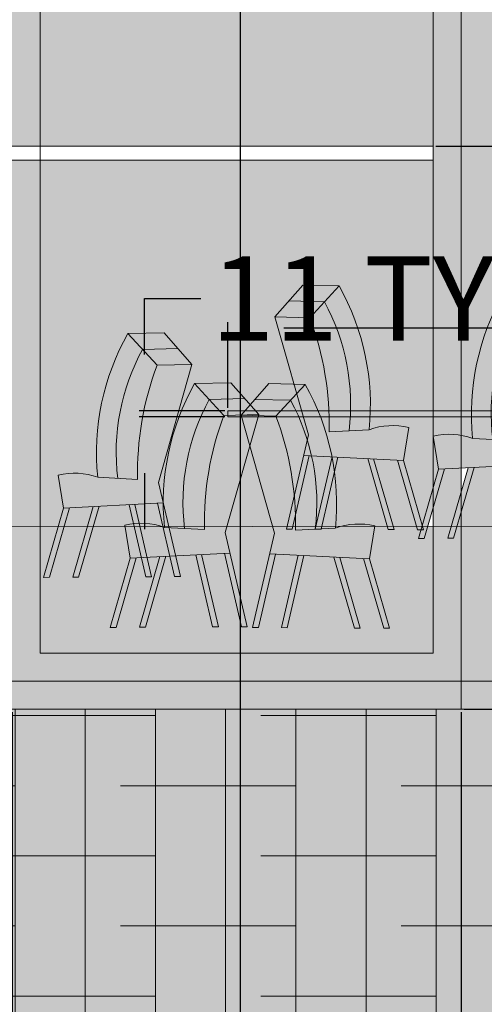
# Model space of a CAD drawing. Units: millimetres. Extents: x 11032 to 26788, y 3406 to 24505.
# Tile 15 of 78: x 18758 to 19586, y 6736 to 8490. Entities that reach past the tile are written whole.
import ezdxf

# ---------------------------------------------------------------- set-up
doc = ezdxf.new("R2010")
doc.units = ezdxf.units.MM
doc.header["$MEASUREMENT"] = 0
for name, color, linetype, lineweight in [('A-ANNO-DIMS', 2, 'Continuous', 18), ('A-FURN', 8, 'Continuous', 13), ('A-FURN-PATT', 8, 'Continuous', 13), ('A-GLAZ', 250, 'Continuous', 20), ('A-WALL-INTR', 8, 'Continuous', 18), ('A-WALL-PLIN-PATT', 253, 'Continuous', 13)]:
    doc.layers.add(name, color=color, linetype=linetype, lineweight=lineweight)
for name, color, linetype, lineweight, true_color in [('A-FNSH-INTR-PATT', 253, 'Continuous', 13, 0xc2b29b), ('A-GLAZ-FRAM-PATT', 250, 'Continuous', 13, 0x262627), ('A-WALL-INTR-PATT', 251, 'Continuous', 13, 0x6c6b6a)]:
    doc.layers.add(name, color=color, linetype=linetype, lineweight=lineweight, true_color=true_color)
doc.styles.get("Standard").update_dxf_attribs({"font": 'arial.ttf'})
doc.dimstyles.get("Standard").update_dxf_attribs({"dimtxt": 150, "dimasz": 100, "dimexe": 10, "dimexo": 5, "dimgap": 5, "dimtad": 0, "dimtih": 1, "dimtoh": 1, "dimdec": 0, "dimzin": 0, "dimdsep": 46, "dimtxsty": 'Standard', "dimcen": 0.09, "dimadec": 0, "dimazin": 0, "dimtfac": 1, "dimtdec": 0, "dimtofl": 0, "dimtmove": 0, "dimatfit": 3, "dimfxl": 1, "dimtolj": 1, "dimtzin": 0, "dimarcsym": 0})

# ---------------------------------------------------------------- blocks, each defined once
blk = doc.blocks.new('DINING-CHAIR-ELEV')
blk.add_line((228.7, 123.4), (51, 132.6))
for points in [[(0, 379.5), (49.4, 435.9), (114.1, 434.5)], [(61.2, 132.1), (30.8, 1.2), (20.5, 1.2), (59.5, 169.3), (0, 379.5), (61.9, 377.9)], [(111.9, 129.5), (82.1, 0.9), (71.8, 1), (101.8, 130)], [(165.3, 126.7), (201.8, 0.3), (212.2, 0.3), (175.8, 126.2)]]:
    blk.add_lwpolyline(points)
for points in [[(218.1, 124), (253.9, 0.1), (264.3, 0), (228.7, 123.4), (238.3, 182.2, 0.148451), (167.5, 178.3), (96.6, 174.5, 0.097012), (61.9, 377.9), (114.1, 434.5, -0.154833), (167.8, 178.5)], [(132, 176.4, 0.156877), (88, 406.2), (24.7, 407.7)]]:
    blk.add_lwpolyline(points, format="xyb")
blk = doc.blocks.new('DINING-TABLE-ELEV')
blk.add_lwpolyline([(0, 0), (986.1, 0), (986.1, 11.1), (0, 11.1)], close=True)
blk = doc.blocks.new('*D18')
at = {"layer": 'A-ANNO-DIMS', "color": 0, "lineweight": -2, "transparency": 16777216}
for p, q in [((19128.8, 7798.4), (19128.8, 7951.3)), ((20114.9, 7798.4), (20114.9, 7951.3)), ((19228.8, 7941.3), (20014.9, 7941.3)), ((20114.9, 7941.3), (20214.9, 7941.3))]:
    blk.add_line(p, q, dxfattribs=at)
at = {"layer": 'A-ANNO-DIMS', "color": 0, "transparency": 16777216}
for points in [[(19228.8, 7958), (19228.8, 7924.7), (19128.8, 7941.3)], [(20014.9, 7958), (20014.9, 7924.7), (20114.9, 7941.3)]]:
    blk.add_solid(points, dxfattribs=at)
at = {"layer": 'Defpoints', "color": 0, "transparency": 16777216}
for p in [(20114.9, 7941.3), (19128.8, 7793.4), (20114.9, 7793.4)]:
    blk.add_point(p, dxfattribs=at)
at = {"layer": 'A-ANNO-DIMS', "color": 0, "transparency": 16777216, "insert": (21221.5, 7941.3), "char_height": 150, "attachment_point": 5}
blk.add_mtext('\\A1;TABLETOP 986 TYP.', dxfattribs=at)
blk = doc.blocks.new('*D19')
at = {"layer": 'A-ANNO-DIMS', "color": 0, "lineweight": -2, "transparency": 16777216}
for p, q in [((18980.9, 7893.4), (18980.9, 7993.4)), ((18980.9, 7993.4), (19080.9, 7993.4)), ((19123.8, 7793.4), (18970.9, 7793.4)), ((19123.8, 7782.3), (18970.9, 7782.3)), ((18980.9, 7682.3), (18980.9, 7582.3))]:
    blk.add_line(p, q, dxfattribs=at)
at = {"layer": 'A-ANNO-DIMS', "color": 0, "transparency": 16777216}
for points in [[(18964.2, 7893.4), (18997.6, 7893.4), (18980.9, 7793.4)], [(18964.2, 7682.3), (18997.6, 7682.3), (18980.9, 7782.3)]]:
    blk.add_solid(points, dxfattribs=at)
at = {"layer": 'Defpoints', "color": 0, "transparency": 16777216}
for p in [(18980.9, 7793.4), (19128.8, 7793.4), (19128.8, 7782.3)]:
    blk.add_point(p, dxfattribs=at)
at = {"layer": 'A-ANNO-DIMS', "color": 0, "transparency": 16777216, "insert": (19443.9, 7993.4), "char_height": 150, "attachment_point": 5}
blk.add_mtext('\\A1;11 TYP.', dxfattribs=at)
blk = doc.blocks.new('*D36')
at = {"layer": 'A-ANNO-DIMS', "color": 0, "lineweight": -2, "transparency": 16777216}
for p, q in [((12301.3, 17115.9), (12301.3, 24416.9)), ((25397.4, 4466.4), (25397.4, 24416.9)), ((12401.3, 24406.9), (18569.2, 24406.9)), ((25297.4, 24406.9), (19129.5, 24406.9))]:
    blk.add_line(p, q, dxfattribs=at)
at = {"layer": 'A-ANNO-DIMS', "color": 0, "transparency": 16777216}
for points in [[(12401.3, 24423.5), (12401.3, 24390.2), (12301.3, 24406.9)], [(25297.4, 24423.5), (25297.4, 24390.2), (25397.4, 24406.9)]]:
    blk.add_solid(points, dxfattribs=at)
at = {"layer": 'Defpoints', "color": 0, "transparency": 16777216}
for p in [(25397.4, 24406.9), (12301.3, 17110.9), (25397.4, 4461.4)]:
    blk.add_point(p, dxfattribs=at)
at = {"layer": 'A-ANNO-DIMS', "color": 0, "transparency": 16777216, "insert": (18849.3, 24406.9), "char_height": 150, "attachment_point": 5}
blk.add_mtext('\\A1;13096', dxfattribs=at)
blk = doc.blocks.new('*D50')
at = {"layer": 'A-ANNO-DIMS', "color": 0, "lineweight": -2, "transparency": 16777216}
for p, q in [((19697.4, 16000.7), (19697.4, 3494.9)), ((17953.5, 10206.4), (17953.5, 3494.9)), ((18053.5, 3504.9), (18603.8, 3504.9)), ((19597.4, 3504.9), (19047, 3504.9))]:
    blk.add_line(p, q, dxfattribs=at)
at = {"layer": 'A-ANNO-DIMS', "color": 0, "transparency": 16777216}
for points in [[(18053.5, 3521.6), (18053.5, 3488.2), (17953.5, 3504.9)], [(19597.4, 3521.6), (19597.4, 3488.2), (19697.4, 3504.9)]]:
    blk.add_solid(points, dxfattribs=at)
at = {"layer": 'Defpoints', "color": 0, "transparency": 16777216}
for p in [(19697.4, 16005.7), (17953.5, 10211.4), (19697.4, 3504.9)]:
    blk.add_point(p, dxfattribs=at)
at = {"layer": 'A-ANNO-DIMS', "color": 0, "transparency": 16777216, "insert": (18825.4, 3504.9), "char_height": 150, "attachment_point": 5}
blk.add_mtext('\\A1;1744', dxfattribs=at)
blk = doc.blocks.new('*D57')
at = {"layer": 'A-ANNO-DIMS', "color": 0, "lineweight": -2, "transparency": 16777216}
for p, q in [((14994.7, 7266.4), (14994.7, 24416.9)), ((20894.7, 7266.4), (20894.7, 24416.9)), ((15094.7, 24406.9), (17716, 24406.9)), ((20794.7, 24406.9), (18173.4, 24406.9))]:
    blk.add_line(p, q, dxfattribs=at)
at = {"layer": 'A-ANNO-DIMS', "color": 0, "transparency": 16777216}
for points in [[(15094.7, 24423.5), (15094.7, 24390.2), (14994.7, 24406.9)], [(20794.7, 24423.5), (20794.7, 24390.2), (20894.7, 24406.9)]]:
    blk.add_solid(points, dxfattribs=at)
at = {"layer": 'Defpoints', "color": 0, "transparency": 16777216}
for p in [(20894.7, 24406.9), (14994.7, 7261.4), (20894.7, 7261.4)]:
    blk.add_point(p, dxfattribs=at)
at = {"layer": 'A-ANNO-DIMS', "color": 0, "transparency": 16777216, "insert": (17944.7, 24406.9), "char_height": 150, "attachment_point": 5}
blk.add_mtext('\\A1;5900', dxfattribs=at)
blk = doc.blocks.new('*D59')
at = {"layer": 'A-ANNO-DIMS', "color": 0, "lineweight": -2, "transparency": 16777216}
for p, q in [((19499.7, 8264.7), (26363.9, 8264.7)), ((26353.9, 8164.7), (26353.9, 7844.7)), ((26353.9, 7361.4), (26353.9, 7681.4)), ((19549.7, 7261.4), (26363.9, 7261.4))]:
    blk.add_line(p, q, dxfattribs=at)
at = {"layer": 'A-ANNO-DIMS', "color": 0, "transparency": 16777216}
for points in [[(26337.2, 8164.7), (26370.6, 8164.7), (26353.9, 8264.7)], [(26337.2, 7361.4), (26370.6, 7361.4), (26353.9, 7261.4)]]:
    blk.add_solid(points, dxfattribs=at)
at = {"layer": 'Defpoints', "color": 0, "transparency": 16777216}
for p in [(19494.7, 8264.7), (26353.9, 8264.7), (19544.7, 7261.4)]:
    blk.add_point(p, dxfattribs=at)
at = {"layer": 'A-ANNO-DIMS', "color": 0, "transparency": 16777216, "insert": (26353.9, 7763), "char_height": 150, "attachment_point": 5}
blk.add_mtext('\\A1;1003.3', dxfattribs=at)
blk = doc.blocks.new('*D64')
at = {"layer": 'A-ANNO-DIMS', "color": 0, "lineweight": -2, "transparency": 16777216}
for p, q in [((18744.7, 7256.4), (18744.7, 3494.9)), ((19544.7, 7256.4), (19544.7, 3494.9)), ((18844.7, 3504.9), (18974.2, 3504.9)), ((19444.7, 3504.9), (19315.3, 3504.9))]:
    blk.add_line(p, q, dxfattribs=at)
at = {"layer": 'A-ANNO-DIMS', "color": 0, "transparency": 16777216}
for points in [[(18844.7, 3521.6), (18844.7, 3488.2), (18744.7, 3504.9)], [(19444.7, 3521.6), (19444.7, 3488.2), (19544.7, 3504.9)]]:
    blk.add_solid(points, dxfattribs=at)
at = {"layer": 'Defpoints', "color": 0, "transparency": 16777216}
for p in [(18744.7, 7261.4), (19544.7, 7261.4), (19544.7, 3504.9)]:
    blk.add_point(p, dxfattribs=at)
at = {"layer": 'A-ANNO-DIMS', "color": 0, "transparency": 16777216, "insert": (19144.7, 3504.9), "char_height": 150, "attachment_point": 5}
blk.add_mtext('\\A1;800', dxfattribs=at)
blk = doc.blocks.new('*D66')
at = {"layer": 'A-ANNO-DIMS', "color": 0, "lineweight": -2, "transparency": 16777216}
for p, q in [((16725.9, 10296), (16725.9, 3494.9)), ((19150.9, 10296), (19150.9, 3494.9)), ((16825.9, 3504.9), (17707.6, 3504.9)), ((19050.9, 3504.9), (18169.3, 3504.9))]:
    blk.add_line(p, q, dxfattribs=at)
at = {"layer": 'A-ANNO-DIMS', "color": 0, "transparency": 16777216}
for points in [[(16825.9, 3521.6), (16825.9, 3488.2), (16725.9, 3504.9)], [(19050.9, 3521.6), (19050.9, 3488.2), (19150.9, 3504.9)]]:
    blk.add_solid(points, dxfattribs=at)
at = {"layer": 'Defpoints', "color": 0, "transparency": 16777216}
for p in [(16725.9, 10301), (19150.9, 10301), (19150.9, 3504.9)]:
    blk.add_point(p, dxfattribs=at)
at = {"layer": 'A-ANNO-DIMS', "color": 0, "transparency": 16777216, "insert": (17938.4, 3504.9), "char_height": 150, "attachment_point": 5}
blk.add_mtext('\\A1;2425', dxfattribs=at)

msp = doc.modelspace()

# ---------------------------------------------------------------- hatches: boundary and pattern name
at = {"layer": 'A-FNSH-INTR-PATT'}
h = msp.add_hatch(dxfattribs=at)
h.set_pattern_fill('AR-SAND', color=256, scale=30, angle=45, style=0)
h.paths.add_polyline_path([(17894.704, 10061.399), (17417.202, 10027.292), (17426.61, 8264.696), (17894.704, 8264.696)])
h.paths.add_polyline_path([(18694.704, 10011.399), (17994.704, 10061.399), (17994.704, 8264.696), (18694.704, 8264.696)])
h.paths.add_polyline_path([(19494.704, 9712.419, 0.04762013), (19003.004, 9961.399), (18794.704, 9961.399), (18794.704, 8264.696), (19494.704, 8264.696)])
at = {"layer": 'A-FURN-PATT'}
h = msp.add_hatch(color=256, dxfattribs=at)
h.set_gradient(color1=(82, 15, 16), color2=(153, 0, 38), name='CURVED')
h.paths.add_polyline_path([(19003.146, 7874.383), (18977.037, 7902.703, 0.15687748), (18933.01, 7672.892), (18968.435, 7670.966, -0.09701208)])
h.paths.add_polyline_path([(19040.326, 7904.234), (18977.037, 7902.703), (19003.146, 7874.383), (19065.05, 7876.04)])
h.paths.add_polyline_path([(19015.601, 7932.429), (18950.929, 7931.023), (18977.037, 7902.703), (19040.326, 7904.234)])
h.paths.add_polyline_path([(19300.945, 7987.51), (19274.836, 7959.19, -0.07933255), (19309.145, 7793.43), (19347.658, 7793.43, 0.13292933)])
h.paths.add_polyline_path([(19327.054, 8015.831), (19300.945, 7987.51, -0.13292933), (19347.658, 7793.43), (19382.824, 7793.43, 0.134919)])
h.paths.add_polyline_path([(19274.836, 7959.19), (19212.932, 7960.847), (19246.92, 7840.817), (19266.818, 7840.385, -0.03021453), (19289.703, 7793.43), (19309.145, 7793.43, 0.07933255)])
h.paths.add_polyline_path([(19300.945, 7987.51), (19237.657, 7989.042), (19212.932, 7960.847), (19274.836, 7959.19)])
h.paths.add_polyline_path([(19327.054, 8015.831), (19262.382, 8017.236), (19237.657, 7989.042), (19300.945, 7987.51)])
h = msp.add_hatch(color=256, dxfattribs=at)
h.set_gradient(color1=(254, 234, 185), color2=(254, 204, 102), name='CURVED')
h.paths.add_polyline_path([(18897.244, 7674.837), (18933.01, 7672.892, -0.15687748), (18977.037, 7902.703), (18950.929, 7931.023, 0.15489802)])
h = msp.add_hatch(color=256, dxfattribs=at)
h.set_gradient(color1=(82, 15, 16), color2=(153, 0, 38), name='CURVED')
h.paths.add_polyline_path([(18897.244, 7674.837), (18933.01, 7672.892, -0.15687748), (18977.037, 7902.703), (18950.929, 7931.023, 0.15489802)])
h = msp.add_hatch(color=256, dxfattribs=at)
h.set_gradient(color1=(82, 15, 16), color2=(153, 0, 38), name='CURVED')
h.paths.add_polyline_path([(19065.05, 7876.04), (19003.146, 7874.383, 0.09701208), (18968.435, 7670.966), (18897.584, 7674.818, 0.14845082), (18826.733, 7678.67), (18836.373, 7619.924), (19014.012, 7629.102), (19005.504, 7665.748)])
h.paths.add_polyline_path([(19096, 7813.441), (19069.892, 7841.762, 0.129191), (19014.012, 7629.102), (19023.82, 7586.852), (19051.589, 7586.881, -0.15468389)])
h.paths.add_polyline_path([(19122.109, 7785.121), (19096, 7813.441, 0.15468389), (19051.589, 7586.881), (19087.296, 7586.918, -0.09456116)])
h.paths.add_polyline_path([(19134.564, 7843.167), (19069.892, 7841.762), (19096, 7813.441), (19159.289, 7814.973)])
h.paths.add_polyline_path([(19159.289, 7814.973), (19096, 7813.441), (19122.109, 7785.121), (19128.812, 7785.301), (19128.812, 7793.43), (19159.737, 7793.43), (19168.958, 7803.946)])
h.paths.add_polyline_path([(19240.709, 7812.065), (19177.421, 7813.596), (19168.958, 7803.946), (19178.18, 7793.43), (19223.53, 7793.43)])
h.paths.add_polyline_path([(19251.689, 7823.975), (19246.92, 7840.817), (19202.145, 7841.791), (19177.421, 7813.596), (19240.709, 7812.065)])
h = msp.add_hatch(color=256, dxfattribs=at)
h.set_gradient(color1=(82, 15, 16), color2=(153, 0, 38), name='HEMISPHERICAL')
h.paths.add_polyline_path([(19013.617, 7586.581, 0.00168564), (19012.835, 7586.841), (18972.503, 7586.799), (18985.177, 7532.205), (19025.754, 7534.301)])
h.paths.add_polyline_path([(19018.73, 7533.938), (19008.164, 7533.392), (18971.826, 7407.487), (18982.249, 7407.539)])
h.paths.add_polyline_path([(18965.902, 7531.209), (18955.336, 7530.663), (18919.71, 7407.228), (18930.133, 7407.28)])
h.paths.add_polyline_path([(18962.239, 7586.788), (18946.129, 7586.771), (18955.336, 7530.663), (18965.902, 7531.209), (18975.033, 7531.681)])
h.paths.add_polyline_path([(18985.177, 7532.205), (18975.033, 7531.681), (18982.992, 7497.396), (18993.246, 7497.447)], flags=17)
h.paths.add_polyline_path([(18972.503, 7586.799), (18962.239, 7586.788), (18975.033, 7531.681), (18985.177, 7532.205)])
h.paths.add_polyline_path([(19014.012, 7629.102), (19005.504, 7665.748), (19065.05, 7876.04), (19003.146, 7874.383, 0.09701208), (18968.435, 7670.966), (18897.584, 7674.818, 0.14845082), (18826.733, 7678.67), (18836.373, 7619.924), (18826.768, 7586.647), (18946.129, 7586.771), (18945.696, 7589.409, -0.14024292), (19012.835, 7586.841), (19016.081, 7586.844, -0.02446541)])
h = msp.add_hatch(color=256, dxfattribs=at)
h.set_gradient(color1=(82, 15, 16), color2=(153, 0, 38), name='HEMISPHERICAL')
h.paths.add_polyline_path([(18837.179, 7586.657), (18826.768, 7586.647), (18800.747, 7496.49), (18811.17, 7496.542)])
h.paths.add_polyline_path([(18889.236, 7586.712), (18878.825, 7586.701), (18852.863, 7496.749), (18863.286, 7496.801)])
h.paths.add_polyline_path([(19124.467, 7576.487), (19168.16, 7730.789), (19152.696, 7785.401), (19183.391, 7784.58), (19184.013, 7786.778), (19122.109, 7785.121, 0.09701208), (19087.398, 7581.705), (19024.218, 7585.14), (19035.898, 7534.825), (19132.975, 7539.841)])
h.paths.add_polyline_path([(19213.879, 7537.94), (19203.735, 7538.464), (19173.23, 7407.063), (19183.484, 7407.012)])
h.paths.add_polyline_path([(19132.975, 7539.841), (19122.83, 7539.317), (19153.225, 7408.389), (19163.48, 7408.44)])
h.paths.add_polyline_path([(19082.253, 7537.22), (19072.109, 7536.696), (19101.955, 7408.134), (19112.209, 7408.185)])
h.paths.add_polyline_path([(19328.545, 7532.016), (19317.979, 7532.562), (19354.46, 7406.162), (19364.883, 7406.111)])
h.paths.add_polyline_path([(19391.013, 7588.032, 0.14845082), (19320.162, 7584.18), (19295.134, 7582.819), (19294.99, 7582.203), (19284.736, 7582.254), (19249.311, 7580.328, 0.01220957), (19249.311, 7606.54), (19243.72, 7582.458), (19233.466, 7582.509), (19247.271, 7641.975, 0.0680716), (19214.6, 7783.745), (19183.391, 7784.58), (19168.16, 7730.789), (19212.242, 7575.11), (19203.735, 7538.464), (19381.373, 7529.286)])
h.paths.add_polyline_path([(19264.6, 7535.319), (19254.456, 7535.844), (19224.5, 7406.808), (19234.754, 7406.757)])
h.paths.add_polyline_path([(19381.373, 7529.286), (19370.808, 7529.832), (19406.576, 7405.903), (19416.999, 7405.852)])
h = msp.add_hatch(color=256, dxfattribs=at)
h.set_gradient(color1=(82, 15, 16), color2=(153, 0, 38), name='HEMISPHERICAL')
h.paths.add_polyline_path([(19168.16, 7730.789), (19152.544, 7785.936), (19122.109, 7785.121, 0.09456116), (19087.296, 7586.918), (19127.433, 7586.96)])
h.paths.add_polyline_path([(19208.862, 7587.045), (19234.525, 7587.072), (19247.271, 7641.975, 0.0680716), (19214.6, 7783.745), (19183.391, 7784.58), (19168.16, 7730.789)])
h = msp.add_hatch(color=256, dxfattribs=at)
h.set_gradient(color1=(82, 15, 16), color2=(153, 0, 38), name='CURVED')
h.paths.add_polyline_path([(19247.271, 7641.975), (19270.45, 7741.82, 0.02831382), (19255.335, 7782.328), (19215.135, 7782.328, -0.06736327)])
h.paths.add_polyline_path([(19294.128, 7782.328), (19263.481, 7782.328), (19272.478, 7750.556), (19270.45, 7741.82, -0.01940924), (19278.122, 7713.179), (19314.548, 7711.297, 0.04279078)])
h = msp.add_hatch(color=256, dxfattribs=at)
h.paths.add_polyline_path([(19168.16, 7730.789), (19127.433, 7586.96), (19208.862, 7587.045)])
h.paths.add_polyline_path([(18889.201, 7622.654), (18846.938, 7620.47), (18837.179, 7586.657), (18878.825, 7586.701)])
h.paths.add_polyline_path([(18953.146, 7625.958), (18899.767, 7623.2), (18889.236, 7586.712), (18946.129, 7586.771), (18945.696, 7589.409, -0.03184825), (18960.996, 7592.142)])
h = msp.add_hatch(color=256, dxfattribs=at)
h.set_gradient(color1=(82, 15, 16), color2=(153, 0, 38), name='HEMISPHERICAL')
h.paths.add_polyline_path([(19278.122, 7713.179), (19274.115, 7713.386), (19249.311, 7606.54, -0.00906061), (19249.433, 7587.087), (19285.302, 7587.125, 0.08318767)])
h.paths.add_polyline_path([(19318.877, 7685.094), (19296.136, 7587.136), (19320.792, 7587.162, 0.05678944)])
h.paths.add_polyline_path([(19314.615, 7710.957, 0.00019976), (19314.548, 7711.297), (19278.122, 7713.179, -0.08318767), (19285.302, 7587.125), (19285.867, 7587.125)])
h = msp.add_hatch(color=256, dxfattribs=at)
h.paths.add_polyline_path([(19378.215, 7708.007), (19324.836, 7710.765), (19318.877, 7685.094, -0.05678944), (19320.792, 7587.162), (19329.538, 7587.171, -0.12791363), (19391.013, 7588.032), (19390.882, 7587.235), (19413.066, 7587.258)])
h.paths.add_polyline_path([(19431.044, 7705.278), (19388.781, 7707.461), (19423.471, 7587.269), (19465.091, 7587.312)])
h.paths.add_polyline_path([(19620.903, 7695.209), (19567.524, 7692.451), (19544.704, 7613.382), (19544.704, 7587.395), (19645.908, 7587.501)])
h.paths.add_polyline_path([(19671.625, 7697.83), (19631.048, 7695.733), (19656.172, 7587.511), (19676.379, 7587.532), (19687.935, 7627.573)])
at = {"layer": 'A-GLAZ-FRAM-PATT'}
h = msp.add_hatch(color=256, dxfattribs=at)
h.paths.add_polyline_path([(17944.704, 7311.399), (16344.704, 7311.399), (16344.704, 7261.399), (17944.704, 7261.399)], flags=17)
h.paths.add_polyline_path([(16344.704, 7311.399), (15045.135, 7311.399, -0.98290472), (20844.273, 7311.399), (19544.704, 7311.399), (19544.704, 7261.399), (20894.704, 7261.399, 0.51484406), (16985.951, 10051.255, 0.32026791), (14994.704, 7261.399), (16344.704, 7261.399)])
h.paths.add_polyline_path([(18744.704, 7311.399), (17944.704, 7311.399), (17944.704, 7261.399), (18744.704, 7261.399)], flags=17)
h.paths.add_polyline_path([(19544.704, 7311.399), (18744.704, 7311.399), (18744.704, 7261.399), (19544.704, 7261.399)], flags=17)
h.paths.add_polyline_path([(18694.704, 7361.399), (17994.704, 7361.399), (17994.704, 7311.399), (18694.704, 7311.399)], flags=17)
h.paths.add_polyline_path([(18744.704, 7361.399), (18694.704, 7361.399), (18694.704, 7311.399), (18744.704, 7311.399)], flags=17)
h.paths.add_polyline_path([(17194.704, 7361.399), (17144.704, 7361.399), (17144.704, 7311.399), (17194.704, 7311.399)], flags=17)
h.paths.add_polyline_path([(17431.432, 7361.399), (17194.704, 7361.399), (17194.704, 7311.399), (17431.699, 7311.399)], flags=17)
h.paths.add_polyline_path([(17894.704, 7361.399), (17431.432, 7361.399), (17431.699, 7311.399), (17894.704, 7311.399)], flags=17)
h.paths.add_polyline_path([(17944.704, 7361.399), (17894.704, 7361.399), (17894.704, 7311.399), (17944.704, 7311.399)], flags=17)
h.paths.add_polyline_path([(17994.704, 7361.399), (17944.704, 7361.399), (17944.704, 7311.399), (17994.704, 7311.399)], flags=17)
h = msp.add_hatch(color=256, dxfattribs=at)
h.paths.add_polyline_path([(16394.704, 9712.419, 0.00513365), (16344.704, 9680.076), (16344.704, 7862.164), (16347.378, 7865.214), (16394.704, 7864.185)])
h.paths.add_polyline_path([(17144.704, 10048.871, 0.02352245), (16886.403, 9961.399), (17094.704, 9961.399), (17094.704, 8264.696), (17144.704, 8264.696)])
h.paths.add_polyline_path([(18794.704, 9961.399), (19003.004, 9961.399, 0.02352245), (18744.704, 10048.871), (18744.704, 8264.696), (18794.704, 8264.696)])
h.paths.add_polyline_path([(19544.704, 9680.076, 0.00513365), (19494.704, 9712.419), (19494.704, 7793.43), (19544.704, 7793.43)])
h = msp.add_hatch(color=256, dxfattribs=at)
h.paths.add_polyline_path([(19990.261, 9317.049, 0.04966763), (19544.704, 9680.076), (19544.704, 7793.43), (19562.845, 7793.43, -0.12577567), (19618.686, 8000.275), (19683.358, 8001.68), (19732.808, 7945.291), (19689.807, 7793.43), (19753.644, 7793.43, -0.09668426), (19805.964, 7950.707), (19870.637, 7952.112), (19920.086, 7895.723), (19891.121, 7793.43), (19990.261, 7793.43)])
h.paths.add_polyline_path([(19494.704, 7793.43), (20114.895, 7793.43), (20114.895, 7782.328), (19382.431, 7782.328, -0.01314801), (19380.738, 7759.644), (19309.547, 7755.774, 0.0123693), (19309.538, 7782.328), (19294.128, 7782.328, -0.11709499), (19320.502, 7584.199), (19243.148, 7579.993), (19243.72, 7582.458), (19233.466, 7582.509), (19247.271, 7641.975, 0.06736327), (19215.135, 7782.328), (19182.753, 7782.328), (19168.16, 7730.789), (19153.566, 7782.328), (19128.812, 7782.328), (19128.812, 7785.301), (19122.109, 7785.121, 0.09701208), (19087.398, 7581.705), (19024.218, 7585.14), (19044.517, 7497.701), (19034.262, 7497.65), (19003.867, 7628.578), (18846.938, 7620.47), (18811.17, 7496.542), (18794.704, 7496.46), (18794.704, 8239.696), (19494.704, 8239.696)])
h = msp.add_hatch(color=256, dxfattribs=at)
h.paths.add_polyline_path([(17944.704, 8239.696), (17894.704, 8239.696), (17894.704, 7796.661), (17944.704, 7796.661)])
h.paths.add_polyline_path([(17994.704, 8239.696), (17944.704, 8239.696), (17944.704, 7796.661), (17994.704, 7796.661)])
h.paths.add_polyline_path([(17944.704, 7785.559), (17894.704, 7785.559), (17894.704, 7361.399), (17944.704, 7361.399)])
h.paths.add_polyline_path([(17994.704, 7785.559), (17944.704, 7785.559), (17944.704, 7361.399), (17994.704, 7361.399)])
h.paths.add_polyline_path([(18744.704, 8239.696), (18694.704, 8239.696), (18694.704, 7361.399), (18744.704, 7361.399)])
h.paths.add_polyline_path([(18794.704, 8239.696), (18744.704, 8239.696), (18744.704, 7311.399), (19544.704, 7311.399), (19544.704, 7613.382), (19531.043, 7566.052), (19520.62, 7566), (19544.704, 7649.444), (19544.704, 7691.272), (19514.696, 7689.722), (19494.704, 7620.453), (19494.704, 7361.399), (18794.704, 7361.399)])
at = {"layer": 'A-WALL-INTR-PATT'}
h = msp.add_hatch(color=256, dxfattribs=at)
h.paths.add_polyline_path([(19494.704, 9712.419, 0.04762013), (19003.004, 9961.399), (18794.704, 9961.399), (18794.704, 8264.696), (19494.704, 8264.696)])
h.paths.add_polyline_path([(18694.704, 10011.399), (17994.704, 10061.399), (17994.704, 8264.696), (18694.704, 8264.696)])
h.paths.add_polyline_path([(17894.704, 10061.399), (17417.202, 10027.292), (17426.61, 8264.696), (17894.704, 8264.696)])
h = msp.add_hatch(color=256, dxfattribs=at)
h.paths.add_polyline_path([(15302.659, 8457.059, 0.02810018), (15185.248, 8153.253), (15233.282, 7717.599), (15314.374, 7311.399), (15467.334, 7311.399), (15381.661, 7740.545)])
h.paths.add_polyline_path([(16344.704, 7543.521), (16344.704, 7643.635), (16302.264, 7793.515), (16205.738, 7793.515), (16227.021, 7719.773), (16216.598, 7719.825), (16195.329, 7793.515), (16153.697, 7793.515), (16174.905, 7720.032), (16164.482, 7720.084), (16143.289, 7793.515), (16061.685, 7793.515), (16051.641, 7750.248, -0.01671442), (16059.629, 7748.571), (16049.99, 7689.825), (16085.615, 7566.39), (16075.192, 7566.442), (16039.424, 7690.371), (15997.161, 7692.554), (16033.5, 7566.649), (16023.077, 7566.701), (15986.595, 7693.1), (15933.216, 7695.858), (15903.371, 7567.296), (15893.116, 7567.347), (15923.072, 7696.382), (15882.495, 7698.478), (15852.409, 7568.882), (15877.716, 7481.201), (15867.293, 7481.253), (15844.553, 7560.041), (15844.691, 7311.399), (16344.704, 7311.399), (16344.704, 7499.3), (16328.717, 7430.435), (16318.463, 7430.486)])
h.paths.add_polyline_path([(16742.983, 7793.515), (16650.704, 7793.515), (16662.994, 7750.932), (16652.571, 7750.983), (16640.296, 7793.515), (16598.663, 7793.515), (16610.879, 7751.191), (16600.455, 7751.242), (16588.255, 7793.515), (16490.425, 7793.515), (16480.749, 7751.837), (16470.495, 7751.888), (16480.159, 7793.515), (16443.833, 7793.515, -0.10940509), (16465.746, 7607.731, -0.14766935), (16536.246, 7611.456), (16526.606, 7552.71), (16562.232, 7429.275), (16551.809, 7429.327), (16516.041, 7553.255), (16473.778, 7555.439), (16510.116, 7429.534), (16499.693, 7429.586), (16463.212, 7555.985), (16409.833, 7558.743), (16394.704, 7493.572), (16394.704, 7361.399), (16744.704, 7361.399)])
h.paths.add_polyline_path([(17094.704, 8239.696), (16741.207, 8239.696), (16742.939, 7804.617), (16768.057, 7804.617), (16785.352, 7864.542), (16775.713, 7923.288, -0.14766935), (16846.212, 7919.563, -0.15483335), (16899.908, 8175.64), (16964.58, 8177.046), (17014.03, 8120.657), (16954.484, 7910.365), (16972.017, 7834.84), (16977.75, 7834.965), (17027.199, 7778.576), (16967.653, 7568.284), (17006.665, 7400.238), (16996.411, 7400.187), (16966.016, 7531.114), (16925.439, 7529.018), (16955.395, 7399.983), (16945.141, 7399.932), (16915.295, 7528.494), (16861.916, 7525.736), (16825.435, 7399.337), (16815.012, 7399.285), (16851.35, 7525.19), (16809.087, 7523.007), (16773.319, 7399.078), (16762.896, 7399.026), (16798.521, 7522.461), (16788.882, 7581.207, -0.14766935), (16859.382, 7577.482, -0.15281323), (16911.41, 7830.579), (16902.125, 7870.575), (16848.746, 7867.817), (16830.506, 7804.617), (16830.506, 7793.515), (16827.302, 7793.515), (16812.265, 7741.418), (16801.842, 7741.366), (16816.893, 7793.515), (16775.261, 7793.515), (16760.15, 7741.159), (16749.727, 7741.107), (16764.853, 7793.515), (16742.983, 7793.515), (16744.704, 7361.399), (17094.704, 7361.399)])
h.paths.add_polyline_path([(18950.929, 7931.023), (19015.601, 7932.429), (19065.05, 7876.04), (19005.504, 7665.748), (19014.012, 7629.102, -0.129191), (19069.892, 7841.762), (19134.564, 7843.167), (19168.958, 7803.946), (19202.145, 7841.791), (19246.92, 7840.817), (19212.932, 7960.847), (19262.382, 8017.236), (19327.054, 8015.831, -0.134919), (19382.824, 7793.43), (19562.845, 7793.43, -0.12577567), (19618.686, 8000.275), (19683.358, 8001.68), (19732.808, 7945.291), (19689.807, 7793.43), (19753.644, 7793.43, -0.09668426), (19805.964, 7950.707), (19870.637, 7952.112), (19920.086, 7895.723), (19891.121, 7793.43), (20039.255, 7793.43, -0.08978651), (20089.9, 7938.993), (20154.572, 7940.399), (20204.021, 7884.01), (20144.475, 7673.718), (20152.983, 7637.072, -0.14766935), (20223.483, 7633.347, -0.15483335), (20277.178, 7889.425), (20341.85, 7890.831), (20391.3, 7834.441), (20331.754, 7624.15), (20370.766, 7456.103), (20360.512, 7456.052), (20330.117, 7586.98), (20289.54, 7584.884), (20319.496, 7455.848), (20309.241, 7455.797), (20279.396, 7584.359), (20226.017, 7581.602), (20189.536, 7455.202), (20179.112, 7455.151), (20215.451, 7581.056), (20173.188, 7578.872), (20169.478, 7566.018), (20183.488, 7505.671), (20173.234, 7505.62), (20163.789, 7546.305), (20137.42, 7454.943), (20126.997, 7454.892), (20159.149, 7566.291), (20142.839, 7636.548), (20102.261, 7634.452), (20132.217, 7505.417), (20121.963, 7505.366), (20092.117, 7633.928), (20038.738, 7631.17), (20002.257, 7504.771), (19991.834, 7504.719), (20028.172, 7630.624), (19985.91, 7628.44), (19950.141, 7504.512), (19939.718, 7504.46), (19975.344, 7627.895), (19965.704, 7686.641, -0.14766935), (20036.204, 7682.916, -0.05764867), (20037.659, 7782.328), (19887.977, 7782.328), (19860.54, 7685.431), (19899.552, 7517.385), (19889.298, 7517.334), (19858.903, 7648.261), (19818.326, 7646.165), (19848.282, 7517.13), (19838.028, 7517.079), (19808.182, 7645.641), (19754.803, 7642.883), (19718.322, 7516.484), (19707.899, 7516.432), (19744.237, 7642.337), (19701.974, 7640.154), (19698.264, 7627.3), (19712.274, 7566.953), (19702.02, 7566.902), (19692.575, 7607.587), (19666.206, 7516.225), (19655.783, 7516.173), (19687.935, 7627.573), (19671.625, 7697.83), (19631.048, 7695.733), (19661.003, 7566.698), (19650.749, 7566.647), (19620.903, 7695.209), (19567.524, 7692.451), (19531.043, 7566.052), (19520.62, 7566), (19556.959, 7691.905), (19514.696, 7689.722), (19478.928, 7565.793), (19468.505, 7565.741), (19473, 7581.318), (19466.812, 7581.349), (19431.044, 7705.278), (19388.781, 7707.461), (19425.12, 7581.556), (19414.696, 7581.608), (19378.215, 7708.007), (19324.836, 7710.765), (19318.877, 7685.094, -0.05845232), (19320.513, 7584.307, -0.14766935), (19391.013, 7588.032), (19381.373, 7529.286), (19416.999, 7405.852), (19406.576, 7405.903), (19370.808, 7529.832), (19328.545, 7532.016), (19364.883, 7406.111), (19354.46, 7406.162), (19317.979, 7532.562), (19264.6, 7535.319), (19234.754, 7406.757), (19224.5, 7406.808), (19254.456, 7535.844), (19213.879, 7537.94), (19183.484, 7407.012), (19173.23, 7407.063), (19212.242, 7575.11), (19168.16, 7730.789), (19124.467, 7576.487), (19163.48, 7408.44), (19153.225, 7408.389), (19122.83, 7539.317), (19082.253, 7537.22), (19112.209, 7408.185), (19101.955, 7408.134), (19072.109, 7536.696), (19035.898, 7534.825), (19044.517, 7497.701), (19034.262, 7497.65), (19025.754, 7534.301), (19018.73, 7533.938), (18982.249, 7407.539), (18971.826, 7407.487), (19008.164, 7533.392), (18985.177, 7532.205), (18993.246, 7497.447), (18982.992, 7497.396), (18975.033, 7531.681), (18965.902, 7531.209), (18930.133, 7407.28), (18919.71, 7407.228), (18955.336, 7530.663), (18945.696, 7589.409, -0.03184825), (18960.996, 7592.142), (18953.146, 7625.958), (18899.767, 7623.2), (18863.286, 7496.801), (18852.863, 7496.749), (18889.201, 7622.654), (18846.938, 7620.47), (18811.17, 7496.542), (18800.747, 7496.49), (18836.373, 7619.924), (18826.733, 7678.67, -0.14766935), (18897.233, 7674.946, -0.15483335)], flags=16)
h = msp.add_hatch(color=256, dxfattribs=at)
h.set_gradient(color1=(254, 234, 185), color2=(254, 204, 102), name='CURVED')
h.paths.add_polyline_path([(15260.167, 7582.928), (15062.56, 7582.722, 0.02345098), (15045.135, 7311.399), (15314.374, 7311.399)])
h.paths.add_polyline_path([(15413.095, 7583.087), (15260.167, 7582.928), (15314.374, 7311.399), (15467.334, 7311.399)])
h.paths.add_polyline_path([(15531.986, 7554.365), (15523.82, 7583.203), (15413.095, 7583.087), (15467.334, 7311.399), (15790.119, 7311.399), (15790.667, 7566.433), (15785.748, 7583.476), (15718.988, 7583.406), (15701.389, 7507.6), (15736.743, 7385.107), (15726.32, 7385.159), (15696.749, 7487.614), (15695.471, 7482.107), (15685.217, 7482.158), (15691.06, 7507.327), (15690.552, 7509.088), (15650.881, 7511.137), (15649.743, 7506.234), (15684.627, 7385.366), (15674.204, 7385.418), (15646.227, 7482.352), (15633.946, 7482.413), (15639.413, 7505.961), (15637.723, 7511.817), (15584.344, 7514.575), (15554.498, 7386.013), (15544.244, 7386.064), (15574.2, 7515.099), (15533.623, 7517.195), (15503.228, 7386.268), (15492.974, 7386.319)])
h.paths.add_polyline_path([(16344.704, 7499.3), (16328.717, 7430.435), (16318.463, 7430.486), (16344.704, 7543.521), (16344.704, 7584.059), (16080.595, 7583.783), (16085.615, 7566.39), (16075.192, 7566.442), (16070.19, 7583.773), (16028.57, 7583.729), (16033.5, 7566.649), (16023.077, 7566.701), (16018.165, 7583.718), (15907.156, 7583.603), (15903.371, 7567.296), (15893.116, 7567.347), (15896.888, 7583.592), (15855.814, 7583.549), (15852.409, 7568.882), (15877.716, 7481.201), (15867.293, 7481.253), (15844.553, 7560.041), (15844.691, 7311.399), (16344.704, 7311.399)])
h.paths.add_polyline_path([(15844.553, 7560.041), (15842.372, 7567.599), (15841.846, 7567.602), (15842.08, 7568.609), (15837.773, 7583.53), (15796.153, 7583.487), (15825.6, 7481.46), (15815.177, 7481.512), (15790.667, 7566.433), (15790.119, 7311.399), (15844.691, 7311.399)])
h.paths.add_polyline_path([(16394.704, 7493.572), (16379.987, 7430.181), (16369.733, 7430.232), (16394.704, 7537.793), (16394.704, 7559.524), (16359.112, 7561.363), (16344.704, 7499.3), (16344.704, 7311.399), (17144.704, 7311.399), (17144.704, 7584.893), (17094.704, 7584.841), (17094.704, 7361.399), (16394.704, 7361.399)])
h.paths.add_polyline_path([(17430.237, 7585.191), (17194.704, 7584.945), (17194.704, 7361.399), (17431.432, 7361.399)])
h.paths.add_polyline_path([(17894.704, 7585.675), (17748.458, 7585.522), (17754.673, 7563.99), (17744.25, 7564.042), (17738.053, 7585.511), (17696.433, 7585.468), (17702.557, 7564.249), (17692.134, 7564.301), (17686.028, 7585.457), (17577.175, 7585.344), (17572.428, 7564.896), (17562.174, 7564.947), (17566.907, 7585.333), (17525.833, 7585.29), (17521.158, 7565.151), (17510.903, 7565.202), (17515.565, 7585.28), (17430.237, 7585.191), (17431.432, 7361.399), (17894.704, 7361.399)])
h.paths.add_polyline_path([(18694.704, 7586.509), (18404.857, 7586.207), (18425.604, 7496.839), (18415.35, 7496.788), (18394.593, 7586.196), (18353.54, 7586.153), (18374.333, 7496.584), (18364.079, 7496.533), (18343.276, 7586.142), (18270.386, 7586.066), (18244.373, 7495.938), (18233.95, 7495.887), (18259.974, 7586.056), (18218.329, 7586.012), (18192.257, 7495.679), (18181.834, 7495.628), (18207.918, 7586.001), (17994.704, 7585.779), (17994.704, 7361.399), (18694.704, 7361.399)])
h.paths.add_polyline_path([(19317.979, 7532.562), (19264.6, 7535.319), (19234.754, 7406.757), (19224.5, 7406.808), (19254.456, 7535.844), (19213.879, 7537.94), (19183.484, 7407.012), (19173.23, 7407.063), (19212.242, 7575.11), (19208.862, 7587.045), (19127.433, 7586.96), (19124.467, 7576.487), (19163.48, 7408.44), (19153.225, 7408.389), (19122.83, 7539.317), (19082.253, 7537.22), (19112.209, 7408.185), (19101.955, 7408.134), (19072.109, 7536.696), (19035.898, 7534.825), (19044.517, 7497.701), (19034.262, 7497.65), (19025.754, 7534.301), (19018.73, 7533.938), (18982.249, 7407.539), (18971.826, 7407.487), (19008.164, 7533.392), (18985.177, 7532.205), (18993.246, 7497.447), (18982.992, 7497.396), (18975.033, 7531.681), (18965.902, 7531.209), (18930.133, 7407.28), (18919.71, 7407.228), (18955.336, 7530.663), (18946.129, 7586.771), (18889.236, 7586.712), (18863.286, 7496.801), (18852.863, 7496.749), (18878.825, 7586.701), (18837.179, 7586.657), (18811.17, 7496.542), (18800.747, 7496.49), (18826.768, 7586.647), (18794.704, 7586.613), (18794.704, 7361.399), (19494.704, 7361.399), (19494.704, 7587.343), (19485.145, 7587.333), (19478.928, 7565.793), (19468.505, 7565.741), (19473, 7581.318), (19466.812, 7581.349), (19465.091, 7587.312), (19423.471, 7587.269), (19425.12, 7581.556), (19414.696, 7581.608), (19413.066, 7587.258), (19390.882, 7587.235), (19381.373, 7529.286), (19416.999, 7405.852), (19406.576, 7405.903), (19370.808, 7529.832), (19328.545, 7532.016), (19364.883, 7406.111), (19354.46, 7406.162)])
h.paths.add_polyline_path([(19990.261, 7587.86), (19974.192, 7587.843), (19950.141, 7504.512), (19939.718, 7504.46), (19963.781, 7587.832), (19883.217, 7587.748), (19899.552, 7517.385), (19889.298, 7517.334), (19872.954, 7587.737), (19831.9, 7587.695), (19848.282, 7517.13), (19838.028, 7517.079), (19821.637, 7587.684), (19738.846, 7587.598), (19718.322, 7516.484), (19707.899, 7516.432), (19728.435, 7587.587), (19707.489, 7587.565), (19712.274, 7566.953), (19702.02, 7566.902), (19697.225, 7587.554), (19686.79, 7587.543), (19666.206, 7516.225), (19655.783, 7516.173), (19676.379, 7587.532), (19656.172, 7587.511), (19661.003, 7566.698), (19650.749, 7566.647), (19645.908, 7587.501), (19544.704, 7587.395), (19544.704, 7311.399), (19990.261, 7311.399)])
h.paths.add_polyline_path([(20190.261, 7455.206), (20179.112, 7455.151), (20190.261, 7493.779), (20190.261, 7579.754), (20173.188, 7578.872), (20169.478, 7566.018), (20183.488, 7505.671), (20173.234, 7505.62), (20163.789, 7546.305), (20137.42, 7454.943), (20126.997, 7454.892), (20159.149, 7566.291), (20154.102, 7588.03), (20113.048, 7587.988), (20132.217, 7505.417), (20121.963, 7505.366), (20102.785, 7587.977), (20026.249, 7587.897), (20002.257, 7504.771), (19990.261, 7504.711), (19990.261, 7311.399), (20190.261, 7311.399)])
h.paths.add_polyline_path([(20340.261, 7543.283), (20330.117, 7586.98), (20289.54, 7584.884), (20319.496, 7455.848), (20309.241, 7455.797), (20279.396, 7584.359), (20226.017, 7581.602), (20190.261, 7457.717), (20190.261, 7311.399), (20340.261, 7311.399)])
h.paths.add_polyline_path([(20826.171, 7588.731), (20340.261, 7588.225), (20340.261, 7587.504), (20370.766, 7456.103), (20360.512, 7456.052), (20340.261, 7543.283), (20340.261, 7311.399), (20844.273, 7311.399, 0.02397257)])
at = {"layer": 'A-WALL-PLIN-PATT'}
h = msp.add_hatch(color=256, dxfattribs=at)
h.set_gradient(color1=(99, 100, 102), color2=(199, 200, 202), name='CYLINDER')
edge = h.paths.add_edge_path()
edge.add_arc((17944.704, 7261.399), 2950, 180, 181.942602)
edge.add_line((14996.399, 7161.399), (12932.665, 7161.399))
edge.add_line((12932.665, 7161.399), (12932.665, 6411.399))
edge.add_line((12932.665, 6411.399), (25397.404, 6411.399))
edge.add_line((25397.404, 6411.399), (25397.404, 7161.399))
edge.add_line((25397.404, 7161.399), (22955.171, 7161.399))
edge.add_spline(control_points=[(22955.171, 7161.399), (22875.95, 7159.113), (22796.729, 7156.828), (22718.347, 7161.399)], knot_values=[0, 0, 0, 0, 236.62389499, 236.62389499, 236.62389499, 236.62389499], degree=3, periodic=0)
edge.add_spline(control_points=[(22718.347, 7161.399), (22709.27, 7161.929), (22517.84, 7175.049), (22332.009, 7233.921), (22155.123, 7291.176)], knot_values=[236.62389499, 236.62389499, 236.62389499, 236.62389499, 264.02785008, 815.24414583, 815.24414583, 815.24414583, 815.24414583], degree=3, periodic=0)
edge.add_line((22155.123, 7291.176), (22155.123, 7161.399))
edge.add_line((22155.123, 7161.399), (20893.008, 7161.399))
edge.add_arc((17944.704, 7261.399), 2950, 358.057398, 360)
edge.add_line((20894.704, 7261.399), (14994.704, 7261.399))
h.paths.add_polyline_path([(14996.399, 6261.399), (14822.389, 6162.807), (21067.019, 6162.807), (20893.008, 6261.399)])
h.paths.add_polyline_path([(14822.224, 6012.807), (14648.718, 5913.331), (21240.69, 5913.331), (21067.183, 6012.807)])
h.paths.add_polyline_path([(21414.634, 5661.399), (21414.635, 5662.395), (21241.977, 5763.336), (14647.43, 5763.336), (14474.772, 5662.395), (14474.774, 5661.399)])
h.paths.add_polyline_path([(14474.964, 5512.395), (14302.433, 5411.236), (21586.974, 5411.236), (21414.443, 5512.395)])
h.paths.add_polyline_path([(14301.435, 5261.24), (14128.313, 5161.097), (21761.094, 5161.097), (21587.972, 5261.24)])
h.paths.add_polyline_path([(22722.526, 4461.399), (21760.979, 5011.097), (14128.428, 5011.097), (13166.882, 4461.399)])
h = msp.add_hatch(dxfattribs=at)
h.set_pattern_fill('ANSI38', color=256, scale=1000, angle=45, style=0)
edge = h.paths.add_edge_path()
edge.add_line((25397.404, 6411.399), (25397.404, 7161.399))
edge.add_line((25397.404, 7161.399), (22955.171, 7161.399))
edge.add_spline(control_points=[(22955.171, 7161.399), (22875.95, 7159.113), (22796.729, 7156.828), (22718.347, 7161.399)], knot_values=[0, 0, 0, 0, 236.62389499, 236.62389499, 236.62389499, 236.62389499], degree=3, periodic=0)
edge.add_spline(control_points=[(22718.347, 7161.399), (22709.27, 7161.929), (22517.84, 7175.049), (22332.009, 7233.921), (22155.123, 7291.176)], knot_values=[236.62389499, 236.62389499, 236.62389499, 236.62389499, 264.02785008, 815.24414583, 815.24414583, 815.24414583, 815.24414583], degree=3, periodic=0)
edge.add_line((22155.123, 7291.176), (22155.123, 7161.399))
edge.add_line((22155.123, 7161.399), (20893.008, 7161.399))
edge.add_arc((17944.704, 7261.399), 2950, 358.057398, 360)
edge.add_line((20894.704, 7261.399), (14994.704, 7261.399))
edge.add_arc((17944.704, 7261.399), 2950, 180, 181.942602)
edge.add_line((14996.399, 7161.399), (12932.665, 7161.399))
edge.add_line((12932.665, 7161.399), (12932.665, 6411.399))
edge.add_line((12932.665, 6411.399), (25397.404, 6411.399))

# ---------------------------------------------------------------- linework, layer by layer
at = {"layer": 'A-GLAZ'}
for p, q in [((18794.704, 7361.399), (18794.704, 9961.399)), ((19494.704, 7361.399), (19494.704, 9712.419)), ((19544.704, 7261.399), (19544.704, 9680.076)), ((18794.704, 7361.399), (19494.704, 7361.399)), ((15045.135, 7311.399), (20844.273, 7311.399)), ((14994.704, 7261.399), (20894.704, 7261.399))]:
    msp.add_line(p, q, dxfattribs=at)
for radius, start, end in [(2950, 358.057398, 108.965621), (2900, 0.987907, 179.012093)]:
    msp.add_arc((17944.704, 7261.399), radius, start, end, dxfattribs=at)
at = {"layer": 'A-WALL-INTR'}
for p, q in [((16741.107, 8264.696), (19494.704, 8264.696)), ((16741.107, 8239.696), (19494.704, 8239.696)), ((15062.56, 7582.722), (20826.171, 7588.731))]:
    msp.add_line(p, q, dxfattribs=at)

# ---------------------------------------------------------------- block references
at = {"layer": 'A-FURN'}
for name, p in [('DINING-CHAIR-ELEV', (19212.932, 7581.297)), ('DINING-CHAIR-ELEV', (19152.696, 7405.852)), ('DINING-TABLE-ELEV', (19128.812, 7782.328))]:
    msp.add_blockref(name, p, dxfattribs=at)
at = {"layer": 'A-FURN', "extrusion": (0, 0, -1), "zscale": -1}
for p in [(-19732.808, 7565.741), (-19065.05, 7496.49), (-19184.013, 7407.228)]:
    msp.add_blockref('DINING-CHAIR-ELEV', p, dxfattribs=at)

# ---------------------------------------------------------------- dimensions: what is measured, and where the dimension line sits
at = {"layer": 'A-ANNO-DIMS'}
for base, p1, p2, picture, middle in [((25397.404, 24406.858), (12301.265, 17110.885), (25397.404, 4461.399), '*D36', (18849.334, 24406.858)), ((20894.704, 24406.858), (14994.704, 7261.399), (20894.704, 7261.399), '*D57', (17944.704, 24406.858)), ((19697.404, 3504.899), (17953.455, 10211.41), (19697.404, 16005.71), '*D50', (18825.429, 3504.899)), ((19150.949, 3504.899), (16725.949, 10301.016), (19150.949, 10301.016), '*D66', (17938.449, 3504.899)), ((19544.704, 3504.899), (18744.704, 7261.399), (19544.704, 7261.399), '*D64', (19144.704, 3504.899))]:
    dim = msp.add_linear_dim(base=base, p1=p1, p2=p2, dimstyle='Standard', override={"dimdec": 0, "dimlfac": 1, "dimrnd": 0, "dimzin": 0, "dimdsep": 46, "dimlunit": 2}, dxfattribs=at)
    dim.commit()
    dim.dimension.update_dxf_attribs({"geometry": picture, "text_midpoint": middle})
dim = msp.add_linear_dim(base=(20114.895, 7941.343), p1=(19128.812, 7793.43), p2=(20114.895, 7793.43), text='TABLETOP <> TYP.', dimstyle='Standard', override={"dimdec": 0, "dimlfac": 1, "dimrnd": 0, "dimzin": 0, "dimdsep": 46, "dimlunit": 2}, dxfattribs=at)
dim.commit()
dim.dimension.update_dxf_attribs({"geometry": '*D18', "text_midpoint": (21221.549, 7941.343)})
dim = msp.add_linear_dim(base=(26353.904, 8264.696), p1=(19544.704, 7261.399), p2=(19494.704, 8264.696), angle=90, dimstyle='Standard', override={"dimdec": 1, "dimlfac": 1, "dimrnd": 0, "dimzin": 0, "dimdsep": 46, "dimlunit": 2}, dxfattribs=at)
dim.commit()
dim.dimension.update_dxf_attribs({"geometry": '*D59', "text_midpoint": (26353.904, 7763.048)})
dim = msp.add_linear_dim(base=(18980.9, 7793.43), p1=(19128.812, 7782.328), p2=(19128.812, 7793.43), angle=90, text='<> TYP.', dimstyle='Standard', override={"dimdec": 0, "dimlfac": 1, "dimrnd": 0, "dimzin": 0, "dimdsep": 46, "dimlunit": 2}, dxfattribs=at)
dim.commit()
dim.dimension.update_dxf_attribs({"geometry": '*D19', "text_midpoint": (19443.915, 7993.43)})

doc.saveas('drawing.dxf')
